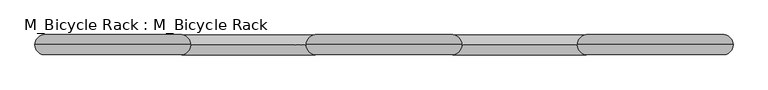
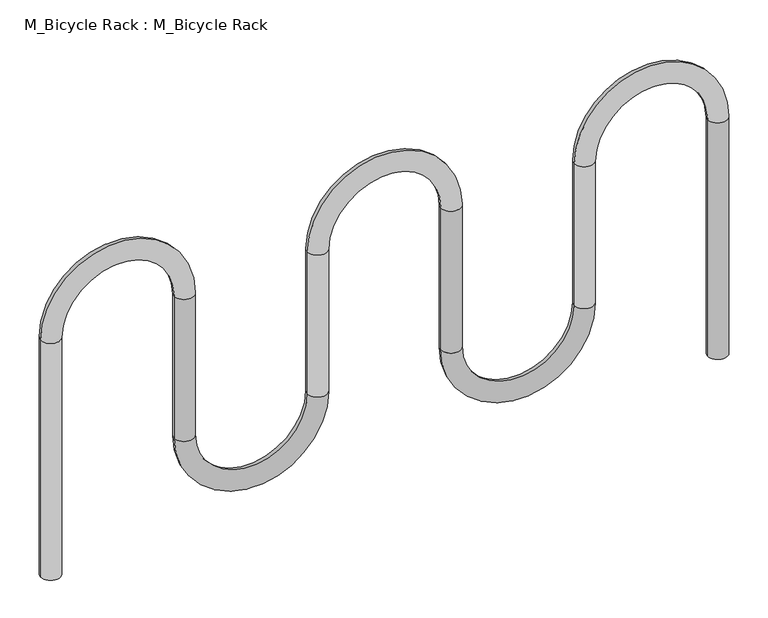
"""IFC4 building model written with IfcOpenShell, lengths in millimetres: proxy geometry, M_Bicycle Rack : M_Bicycle Rack."""

from ifc_helpers import new_model, si_unit, point, frame, origin, place, context, project, spatial, circle_curve, ellipse_curve, trimmed, source, transform, mapped, element, save
from ifc_brep_helpers import plane_surface, cylinder_surface, revolved_surface, advanced_brep


def m_bicycle_rack_m_bicycle_rack_69598307(model_context):
    return source(origin(), model_context, "Body", "AdvancedBrep", [
        advanced_brep(
        [(-985.8375, 0.0, 0.0), (-1046.1625, 0.0, 0.0), (-985.8375, 0.0, 762.0), (-1046.1625, 0.0, 762.0), (-579.4375, 0.0, 762.0), (-639.7625, 0.0, 762.0), (-639.7625, 0.0, 304.8), (-579.4375, 0.0, 304.8), (-233.3625, 0.0, 304.8), (-173.0375, 0.0, 304.8), (-173.0375, 0.0, 762.0), (-233.3625, 0.0, 762.0), (233.3625, 0.0, 762.0), (173.0375, 0.0, 762.0), (173.0375, 0.0, 304.8), (233.3625, 0.0, 304.8), (579.4375, 0.0, 304.8), (639.7625, 0.0, 304.8), (639.7625, 0.0, 762.0), (579.4375, 0.0, 762.0), (1046.1625, 0.0, 762.0), (985.8375, 0.0, 762.0), (985.8375, 0.0, 0.0), (1046.1625, 0.0, 0.0)],
        [
            (0, 1, circle_curve(frame((-1016.0, 0.0, 0.0), z_axis=(0.0, 0.0, -1.0), x_axis=(-1.0, 0.0, 0.0)), 30.1625)),
            (1, 0, circle_curve(frame((-1016.0, 0.0, 0.0), z_axis=(0.0, 0.0, -1.0), x_axis=(-1.0, 0.0, 0.0)), 30.1625)),
            (0, 2),
            (2, 3, circle_curve(frame((-1016.0, 0.0, 762.0), z_axis=(0.0, 0.0, -1.0), x_axis=(-1.0, 0.0, 0.0)), 30.1625)),
            (3, 1),
            (3, 2, circle_curve(frame((-1016.0, 0.0, 762.0), z_axis=(0.0, 0.0, -1.0), x_axis=(-1.0, 0.0, 0.0)), 30.1625)),
            (4, 3, circle_curve(frame((-812.8, 0.0, 762.0), z_axis=(0.0, -1.0, 0.0), x_axis=(-1.0, 0.0, 0.0)), 233.3625)),
            (2, 5, circle_curve(frame((-812.8, 0.0, 762.0), z_axis=(0.0, 1.0, 0.0), x_axis=(-1.0, 0.0, 0.0)), 173.0375)),
            (5, 4, circle_curve(frame((-609.6, 0.0, 762.0), z_axis=(0.0, 0.0, 1.0), x_axis=(1.0, 0.0, 0.0)), 30.1625)),
            (4, 5, circle_curve(frame((-609.6, 0.0, 762.0), z_axis=(0.0, 0.0, 1.0), x_axis=(1.0, 0.0, 0.0)), 30.1625)),
            (5, 6),
            (6, 7, circle_curve(frame((-609.6, 0.0, 304.8), z_axis=(0.0, 0.0, 1.0), x_axis=(1.0, 0.0, 0.0)), 30.1625)),
            (7, 4),
            (7, 6, circle_curve(frame((-609.6, 0.0, 304.8), z_axis=(0.0, 0.0, 1.0), x_axis=(1.0, 0.0, 0.0)), 30.1625)),
            (8, 7, circle_curve(frame((-406.4, 0.0, 304.8), z_axis=(0.0, 1.0, 0.0), x_axis=(-1.0, 0.0, 0.0)), 173.0375)),
            (6, 9, circle_curve(frame((-406.4, 0.0, 304.8), z_axis=(0.0, -1.0, 0.0), x_axis=(-1.0, 0.0, 0.0)), 233.3625)),
            (9, 8, circle_curve(frame((-203.2, 0.0, 304.8), z_axis=(0.0, 0.0, -1.0), x_axis=(-1.0, 0.0, 0.0)), 30.1625)),
            (8, 9, circle_curve(frame((-203.2, 0.0, 304.8), z_axis=(0.0, 0.0, -1.0), x_axis=(-1.0, 0.0, 0.0)), 30.1625)),
            (9, 10),
            (10, 11, circle_curve(frame((-203.2, 0.0, 762.0), z_axis=(0.0, 0.0, -1.0), x_axis=(-1.0, 0.0, 0.0)), 30.1625)),
            (11, 8),
            (11, 10, circle_curve(frame((-203.2, 0.0, 762.0), z_axis=(0.0, 0.0, -1.0), x_axis=(-1.0, 0.0, 0.0)), 30.1625)),
            (12, 11, circle_curve(frame((0.0, 0.0, 762.0), z_axis=(0.0, -1.0, 0.0), x_axis=(-1.0, 0.0, 0.0)), 233.3625)),
            (10, 13, circle_curve(frame((0.0, 0.0, 762.0), z_axis=(0.0, 1.0, 0.0), x_axis=(-1.0, 0.0, 0.0)), 173.0375)),
            (13, 12, circle_curve(frame((203.2, 0.0, 762.0), z_axis=(0.0, 0.0, 1.0), x_axis=(1.0, 0.0, 0.0)), 30.1625)),
            (12, 13, circle_curve(frame((203.2, 0.0, 762.0), z_axis=(0.0, 0.0, 1.0), x_axis=(1.0, 0.0, 0.0)), 30.1625)),
            (13, 14),
            (14, 15, circle_curve(frame((203.2, 0.0, 304.8), z_axis=(0.0, 0.0, 1.0), x_axis=(1.0, 0.0, 0.0)), 30.1625)),
            (15, 12),
            (15, 14, circle_curve(frame((203.2, 0.0, 304.8), z_axis=(0.0, 0.0, 1.0), x_axis=(1.0, 0.0, 0.0)), 30.1625)),
            (16, 15, circle_curve(frame((406.4, 0.0, 304.8), z_axis=(0.0, 1.0, 0.0), x_axis=(-1.0, 0.0, 0.0)), 173.0375)),
            (14, 17, circle_curve(frame((406.4, 0.0, 304.8), z_axis=(0.0, -1.0, 0.0), x_axis=(-1.0, 0.0, 0.0)), 233.3625)),
            (17, 16, circle_curve(frame((609.6, 0.0, 304.8), z_axis=(0.0, 0.0, -1.0), x_axis=(-1.0, 0.0, 0.0)), 30.1625)),
            (16, 17, circle_curve(frame((609.6, 0.0, 304.8), z_axis=(0.0, 0.0, -1.0), x_axis=(-1.0, 0.0, 0.0)), 30.1625)),
            (17, 18),
            (18, 19, circle_curve(frame((609.6, 0.0, 762.0), z_axis=(0.0, 0.0, -1.0), x_axis=(-1.0, 0.0, 0.0)), 30.1625)),
            (19, 16),
            (19, 18, circle_curve(frame((609.6, 0.0, 762.0), z_axis=(0.0, 0.0, -1.0), x_axis=(-1.0, 0.0, 0.0)), 30.1625)),
            (20, 19, circle_curve(frame((812.8, 0.0, 762.0), z_axis=(0.0, -1.0, 0.0), x_axis=(-1.0, 0.0, 0.0)), 233.3625)),
            (18, 21, circle_curve(frame((812.8, 0.0, 762.0), z_axis=(0.0, 1.0, 0.0), x_axis=(-1.0, 0.0, 0.0)), 173.0375)),
            (21, 20, circle_curve(frame((1016.0, 0.0, 762.0), z_axis=(0.0, 0.0, 1.0), x_axis=(1.0, 0.0, 0.0)), 30.1625)),
            (20, 21, circle_curve(frame((1016.0, 0.0, 762.0), z_axis=(0.0, 0.0, 1.0), x_axis=(1.0, 0.0, 0.0)), 30.1625)),
            (22, 23, circle_curve(frame((1016.0, 0.0, 0.0), z_axis=(0.0, 0.0, -1.0), x_axis=(1.0, 0.0, 0.0)), 30.1625)),
            (23, 22, circle_curve(frame((1016.0, 0.0, 0.0), z_axis=(0.0, 0.0, -1.0), x_axis=(1.0, 0.0, 0.0)), 30.1625)),
            (21, 22),
            (23, 20),
        ],
        [
            plane_surface(frame((-1016.0, 0.0, 0.0), z_axis=(0.0, 0.0, -1.0), x_axis=(0.0, -1.0, 0.0))),
            cylinder_surface(frame((-1016.0, 0.0, 0.0), z_axis=(0.0, 0.0, -1.0), x_axis=(-1.0, 0.0, 0.0)), 30.1625),
            revolved_surface(trimmed(ellipse_curve(frame((-1016.0, 0.0, 762.0), z_axis=(0.0, 0.0, -1.0), x_axis=(-1.0, 0.0, 0.0)), 30.1625, 30.1625), [point((-985.8375, 0.0, 762.0))], [point((-1046.1625, 0.0, 762.0))], True, "CARTESIAN"), (-812.8, 0.0, 762.0), (0.0, 1.0, 0.0)),
            revolved_surface(trimmed(ellipse_curve(frame((-1016.0, 0.0, 762.0), z_axis=(0.0, 0.0, -1.0), x_axis=(-1.0, 0.0, 0.0)), 30.1625, 30.1625), [point((-1046.1625, 0.0, 762.0))], [point((-985.8375, 0.0, 762.0))], True, "CARTESIAN"), (-812.8, 0.0, 762.0), (0.0, 1.0, 0.0)),
            cylinder_surface(frame((-609.6, 0.0, 762.0), z_axis=(0.0, 0.0, 1.0), x_axis=(1.0, 0.0, 0.0)), 30.1625),
            revolved_surface(trimmed(ellipse_curve(frame((-609.6, 0.0, 304.8), z_axis=(0.0, 0.0, 1.0), x_axis=(1.0, 0.0, 0.0)), 30.1625, 30.1625), [point((-639.7625, 0.0, 304.8))], [point((-579.4375, 0.0, 304.8))], True, "CARTESIAN"), (-406.4, 0.0, 304.8), (0.0, -1.0, 0.0)),
            revolved_surface(trimmed(ellipse_curve(frame((-609.6, 0.0, 304.8), z_axis=(0.0, 0.0, 1.0), x_axis=(1.0, 0.0, 0.0)), 30.1625, 30.1625), [point((-579.4375, 0.0, 304.8))], [point((-639.7625, 0.0, 304.8))], True, "CARTESIAN"), (-406.4, 0.0, 304.8), (0.0, -1.0, 0.0)),
            cylinder_surface(frame((-203.2, 0.0, 304.8), z_axis=(0.0, 0.0, -1.0), x_axis=(-1.0, 0.0, 0.0)), 30.1625),
            revolved_surface(trimmed(ellipse_curve(frame((-203.2, 0.0, 762.0), z_axis=(0.0, 0.0, -1.0), x_axis=(-1.0, 0.0, 0.0)), 30.1625, 30.1625), [point((-173.0375, 0.0, 762.0))], [point((-233.3625, 0.0, 762.0))], True, "CARTESIAN"), (0.0, 0.0, 762.0), (0.0, 1.0, 0.0)),
            revolved_surface(trimmed(ellipse_curve(frame((-203.2, 0.0, 762.0), z_axis=(0.0, 0.0, -1.0), x_axis=(-1.0, 0.0, 0.0)), 30.1625, 30.1625), [point((-233.3625, 0.0, 762.0))], [point((-173.0375, 0.0, 762.0))], True, "CARTESIAN"), (0.0, 0.0, 762.0), (0.0, 1.0, 0.0)),
            cylinder_surface(frame((203.2, 0.0, 762.0), z_axis=(0.0, 0.0, 1.0), x_axis=(1.0, 0.0, 0.0)), 30.1625),
            revolved_surface(trimmed(ellipse_curve(frame((203.2, 0.0, 304.8), z_axis=(0.0, 0.0, 1.0), x_axis=(1.0, 0.0, 0.0)), 30.1625, 30.1625), [point((173.0375, 0.0, 304.8))], [point((233.3625, 0.0, 304.8))], True, "CARTESIAN"), (406.4, 0.0, 304.8), (0.0, -1.0, 0.0)),
            revolved_surface(trimmed(ellipse_curve(frame((203.2, 0.0, 304.8), z_axis=(0.0, 0.0, 1.0), x_axis=(1.0, 0.0, 0.0)), 30.1625, 30.1625), [point((233.3625, 0.0, 304.8))], [point((173.0375, 0.0, 304.8))], True, "CARTESIAN"), (406.4, 0.0, 304.8), (0.0, -1.0, 0.0)),
            cylinder_surface(frame((609.6, 0.0, 304.8), z_axis=(0.0, 0.0, -1.0), x_axis=(-1.0, 0.0, 0.0)), 30.1625),
            revolved_surface(trimmed(ellipse_curve(frame((609.6, 0.0, 762.0), z_axis=(0.0, 0.0, -1.0), x_axis=(-1.0, 0.0, 0.0)), 30.1625, 30.1625), [point((639.7625, 0.0, 762.0))], [point((579.4375, 0.0, 762.0))], True, "CARTESIAN"), (812.8, 0.0, 762.0), (0.0, 1.0, 0.0)),
            revolved_surface(trimmed(ellipse_curve(frame((609.6, 0.0, 762.0), z_axis=(0.0, 0.0, -1.0), x_axis=(-1.0, 0.0, 0.0)), 30.1625, 30.1625), [point((579.4375, 0.0, 762.0))], [point((639.7625, 0.0, 762.0))], True, "CARTESIAN"), (812.8, 0.0, 762.0), (0.0, 1.0, 0.0)),
            plane_surface(frame((1016.0, 0.0, 0.0), z_axis=(0.0, 0.0, -1.0), x_axis=(0.0, -1.0, 0.0))),
            cylinder_surface(frame((1016.0, 0.0, 762.0), z_axis=(0.0, 0.0, 1.0), x_axis=(1.0, 0.0, 0.0)), 30.1625),
        ],
        [
            (0, [[1, 2]]),
            (1, [[-1, 3, 4, 5]]),
            (1, [[-2, -5, 6, -3]]),
            (2, [[7, -4, 8, 9]]),
            (3, [[-8, -6, -7, 10]]),
            (4, [[-9, 11, 12, 13]]),
            (4, [[-10, -13, 14, -11]]),
            (5, [[15, -12, 16, 17]]),
            (6, [[-16, -14, -15, 18]]),
            (7, [[-17, 19, 20, 21]]),
            (7, [[-18, -21, 22, -19]]),
            (8, [[23, -20, 24, 25]]),
            (9, [[-24, -22, -23, 26]]),
            (10, [[-25, 27, 28, 29]]),
            (10, [[-26, -29, 30, -27]]),
            (11, [[31, -28, 32, 33]]),
            (12, [[-32, -30, -31, 34]]),
            (13, [[-33, 35, 36, 37]]),
            (13, [[-34, -37, 38, -35]]),
            (14, [[39, -36, 40, 41]]),
            (15, [[-40, -38, -39, 42]]),
            (16, [[43, 44]]),
            (17, [[-41, 45, -44, 46]]),
            (17, [[-42, -46, -43, -45]]),
        ],
    ),
    ])


if __name__ == "__main__":
    model = new_model("IFC4")
    model_context = context("Model", 3, world=origin())
    ifc_project = project(units=[si_unit("LENGTHUNIT", "METRE", prefix="MILLI")], contexts=[model_context])
    site = spatial("IfcSite", under=ifc_project)
    building = spatial("IfcBuilding", under=site)
    placement = place(None, origin())
    m_bicycle_rack_m_bicycle_rack_shape = m_bicycle_rack_m_bicycle_rack_69598307(model_context)
    element("IfcBuildingElementProxy", 1, Name="M_Bicycle Rack : M_Bicycle Rack", ObjectType="M_Bicycle Rack : M_Bicycle Rack", at=placement, inside=building, context=model_context, shape_type="MappedRepresentation", body=[
        mapped(m_bicycle_rack_m_bicycle_rack_shape, transform((0.0, 0.0, 0.0), x_axis=(1.0, 0.0, 0.0), y_axis=(0.0, 1.0, 0.0), z_axis=(0.0, 0.0, 1.0))),
    ])
    save(model, "model.ifc")

# Revit data of these elements
# Type "M_Bicycle Rack : M_Bicycle Rack"
#   Default Elevation = 0
